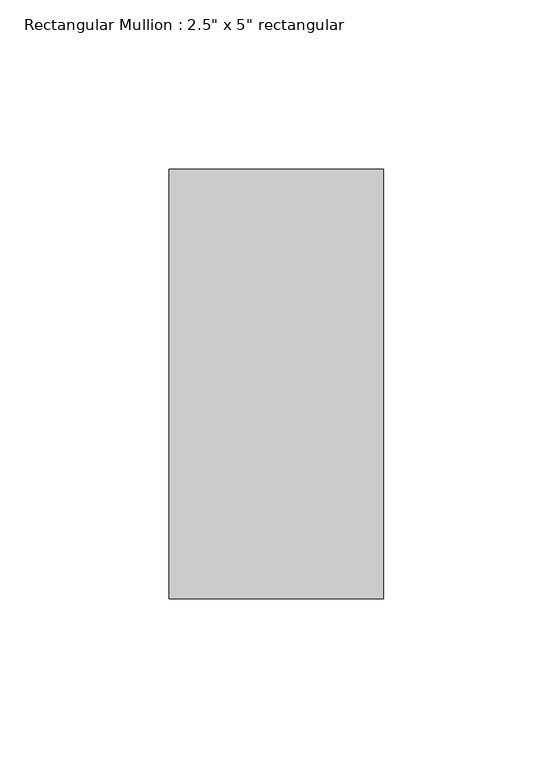
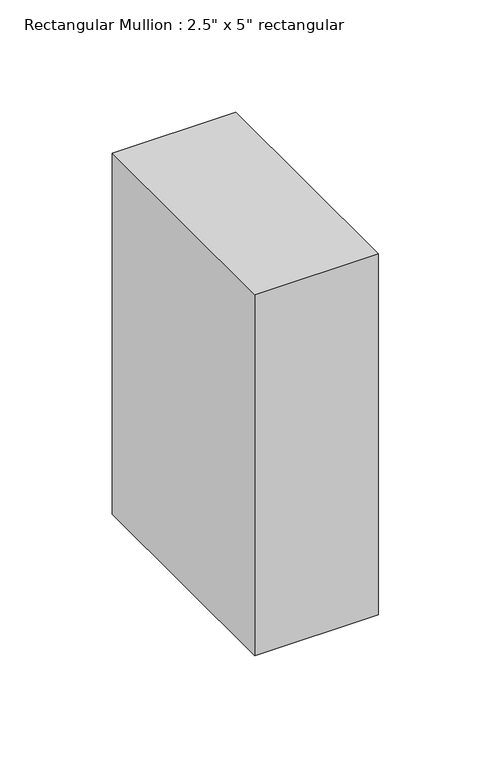
"""IFC4 building model written with IfcOpenShell, lengths in millimetres: member geometry."""

from ifc_helpers import new_model, si_unit, frame, origin, place, context, project, spatial, polyline, outline, extrude, source, transform, mapped, element, save


def member_d97a949f(model_context):
    return source(origin(), model_context, "Body", "SweptSolid", [
        extrude(outline(polyline([(31.75, 63.5), (31.75, -63.5), (-31.75, -63.5), (-31.75, 63.5), (31.75, 63.5)])), frame((0.0, 0.0, -196.1049185), z_axis=(0.0, 0.0, 1.0), x_axis=(1.0, 0.0, 0.0)), (0.0, 0.0, 1.0), 196.1049185),
    ])


if __name__ == "__main__":
    model = new_model("IFC4")
    model_context = context("Model", 3, world=origin())
    ifc_project = project(units=[si_unit("LENGTHUNIT", "METRE", prefix="MILLI")], contexts=[model_context])
    site = spatial("IfcSite", under=ifc_project)
    building = spatial("IfcBuilding", under=site)
    placement = place(None, origin())
    member_shape = member_d97a949f(model_context)
    element("IfcMember", 1, ObjectType="Rectangular Mullion : 2.5\" x 5\" rectangular", at=placement, inside=building, context=model_context, shape_type="MappedRepresentation", body=[
        mapped(member_shape, transform((0.0, 0.0, 0.0), x_axis=(1.0, 0.0, 0.0), y_axis=(0.0, 1.0, 0.0), z_axis=(0.0, 0.0, 1.0))),
    ])
    save(model, "model.ifc")

# Revit data of these elements
# Type "Rectangular Mullion : 2.5\" x 5\" rectangular"
#   built-in parameter 1007304 = 0.416667 (stored number, unit not read)
#   built-in parameter 1007301 = 0.104167 (stored number, unit not read)
#   built-in parameter 1007300 = 0.104167 (stored number, unit not read)
# Element 1 (IfcMember, "Rectangular Mullion : 2.5\" x 5\" rectangular")
#   Materials on its faces: "mullions"
# Materials
#   "mullions": class "Generic", colour RGB 120 120 120, transparency 0, Cost = 0
